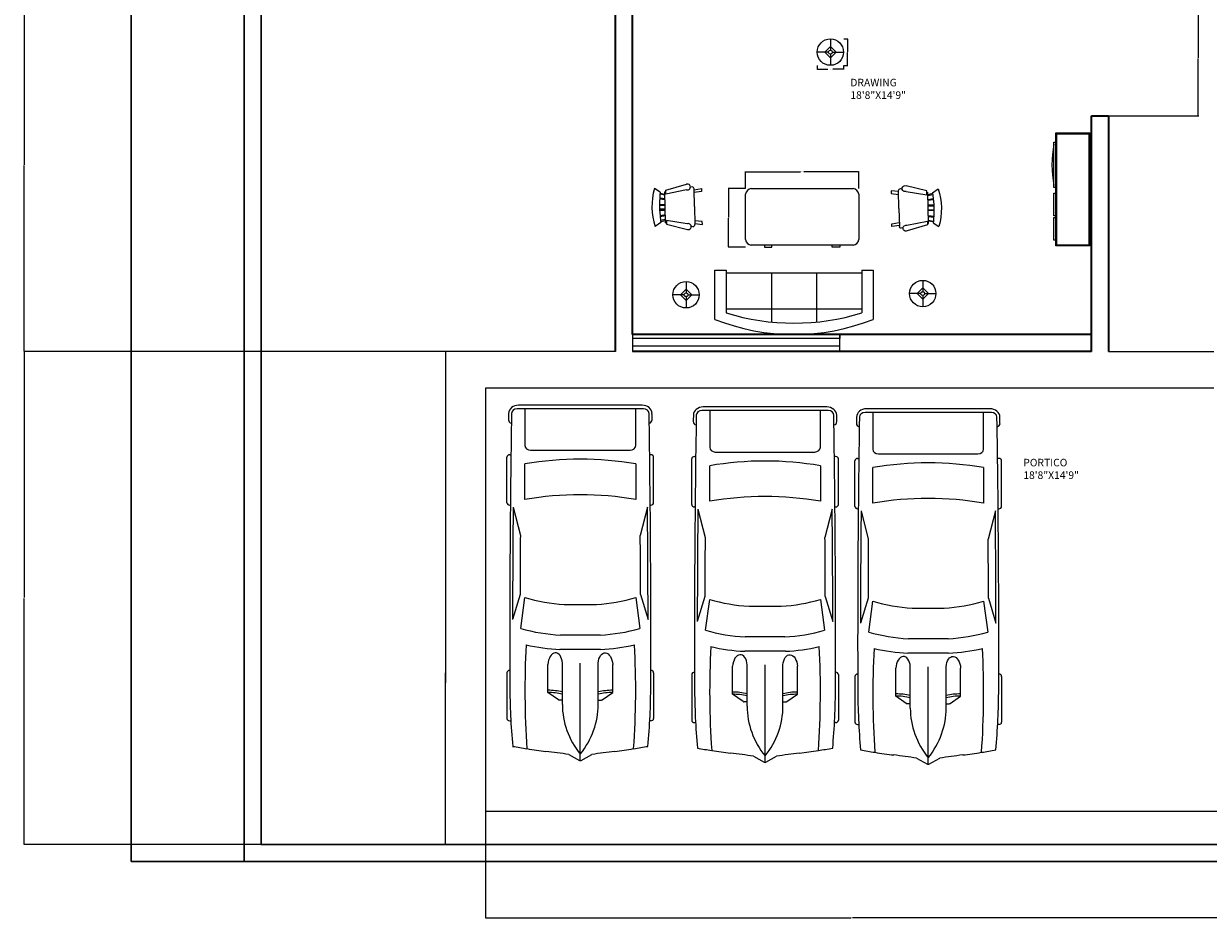
# Model space of a CAD drawing. Units: inches. Extents: x 727 to 1967, y -579 to 606.
# Tile 1 of 5: x 727 to 1355, y -552 to -78. Entities that reach past the tile are written whole.
import ezdxf

# ---------------------------------------------------------------- set-up
doc = ezdxf.new("R2010")
doc.units = ezdxf.units.IN
doc.header["$MEASUREMENT"] = 0
for name, color, linetype, lineweight in [('A-ANNO-DIMS', 2, 'Continuous', 18), ('A-AREA-IDEN', 7, 'Continuous', 18), ('A-FLOR-EXT', 7, 'Continuous', 25), ('A-FURN', 8, 'Continuous', 18), ('A-GLAZ', 4, 'Continuous', 18), ('A-WALL', 7, 'Continuous', 35), ('C-PKNG-VEHI', 8, 'Continuous', 13), ('C-PROP', 7, 'Continuous', 30)]:
    doc.layers.add(name, color=color, linetype=linetype, lineweight=lineweight)
doc.styles.get("Standard").update_dxf_attribs({"font": 'arial.ttf'})
doc.dimstyles.get("Standard").update_dxf_attribs({"dimtxt": 0.18, "dimasz": 0.18, "dimexe": 0.18, "dimexo": 0.0625, "dimgap": 0.09, "dimtad": 0, "dimtih": 1, "dimtoh": 1, "dimdec": 4, "dimzin": 0, "dimdsep": 46, "dimtxsty": 'Standard', "dimcen": 0.09, "dimadec": 0, "dimazin": 0, "dimtfac": 1, "dimtdec": 4, "dimtofl": 0, "dimtmove": 0, "dimatfit": 3, "dimfxl": 1, "dimtolj": 1, "dimtzin": 0, "dimarcsym": 0})

# ---------------------------------------------------------------- blocks, each defined once
blk = doc.blocks.new('Sofa - Roundback 7 ft.')
for p, q in [((-36.000027, -34), (-36.000027, -11.4696)), ((-12.00002, -32.4421), (-12.00003, -6.5971)), ((11.99997, -32.4421), (11.99998, -6.5971)), ((35.99998, -34), (35.99998, -11.4696)), ((-35.999844, -13.3819), (35.9998, -13.3819)), ((-36.000027, -32.4421), (35.99998, -32.4421))]:
    blk.add_line(p, q)
for points in [[(-36.000027, -34), (-42.000027, -34), (-42.000027, -8)], [(41.99998, -8), (41.99998, -34), (35.99998, -34)]]:
    blk.add_lwpolyline(points)
for centre, radius, start, end in [((0, -114.25), 114.25, 68.43141, 111.5686), ((-0.00001, -127.1968), 121.1968, 72.72033, 107.2797)]:
    blk.add_arc(centre, radius, start, end)
blk = doc.blocks.new('Chair - Rocking')
for p, q in [((-8, -4.5), (-10, -1.5)), ((-7.5, -4.5), (-7, -7)), ((-6.5, -7), (-7.02225, -4.43)), ((-4.5, -7), (-4.96674, -4.19951)), ((-4, -7), (-4.40532, -4.16272)), ((-1.5, -4.05012), (-1.5, -7)), ((-1, -7), (-1, -4.05012)), ((1, -7), (1, -4.04655)), ((1.5, -4.05012), (1.5, -7)), ((4, -7), (4.40187, -4.18694)), ((4.5, -7), (4.96761, -4.19437)), ((6.5, -7), (7, -4.4057)), ((7.5, -4.5), (7, -7)), ((8, -4.5), (10, -1.5)), ((-9, -7.5), (-12, -18.49999)), ((-7, -7.5), (-9, -7.5)), ((-9, -18.49999), (-7, -7.5)), ((-8.23428, -6.99939), (-8.3093, -7.47958)), ((-8.23041, -7), (8.23915, -7)), ((7, -7.5), (9, -7.5)), ((9, -18.49999), (7, -7.5)), ((8.31071, -7.48854), (8.23449, -7.00073)), ((9, -7.5), (12, -18.49999)), ((-10.36644, -20.64523), (-10.5, -21.49999)), ((-9, -22.49999), (-9.5, -26.49999)), ((0, -22.49999), (-9.5, -22.49999)), ((-8, -26.49999), (-7.5, -22.49999)), ((0, -22.49999), (9.5, -22.49999)), ((8, -26.49999), (7.5, -22.49999)), ((9, -22.49999), (9.5, -26.49999)), ((10.5, -21.49999), (10.3575, -20.58798)), ((-9.5, -26.49999), (-8, -26.49999)), ((9.5, -26.49999), (8, -26.49999))]:
    blk.add_line(p, q)
for centre, radius, start, end in [((0, -34.08333), 34.08333, 72.93847, 107.0615), ((0, -68.25004), 64.25, 93.92211, 97.15267), ((0, -68.25004), 64.25, 82.84733, 93.92211), ((-10.5, -18.99999), 1.58114, 161.5651, 18.43495), ((10.5, -18.99999), 1.58114, 161.5651, 18.43495), ((-9.5, -21.49999), 1, 180, 270), ((9.5, -21.49999), 1, 270, 0)]:
    blk.add_arc(centre, radius, start, end)
blk = doc.blocks.new('Lamp - Table')
for p, q in [((0, 7), (0, 1)), ((-1, 0), (-7, 0)), ((0, 3), (-3, 0)), ((-3, 0), (0, -3)), ((3, 0), (0, 3)), ((0, -3), (3, 0)), ((1, 0), (7, 0)), ((0, -1), (0, -7))]:
    blk.add_line(p, q)
for radius in [7, 1]:
    blk.add_circle((0, 0), radius)
blk = doc.blocks.new('Entertainment Center')
for p, q in [((-4, 0), (-5, -1)), ((4, 0), (-4, 0)), ((5, -1), (4, 0)), ((-17, -19), (-17, -1)), ((-17, -1), (43, -1)), ((-16.5, -18.5), (-16.5, -1.5)), ((-16.5, -1.5), (42.5, -1.5)), ((42.5, -1.5), (42.5, -18.5)), ((43, -1), (43, -19)), ((42.5, -18.5), (-16.5, -18.5)), ((43, -19), (-17, -19)), ((-12, -20), (-12, -19)), ((12, -20), (-12, -20)), ((12, -19), (12, -20)), ((15, -20), (15, -19)), ((27, -20), (15, -20)), ((27, -19), (27, -20)), ((28, -20), (28, -19)), ((40, -20), (28, -20)), ((40, -19), (40, -20))]:
    blk.add_line(p, q)
blk.add_arc((0, 40), 61, 259.6111, 280.3889)
blk = doc.blocks.new('Desk - 30 x 60 in.')
for p, q in [((-26.999995, 0), (26.999995, 0)), ((-29.999995, -27), (-29.999995, -3)), ((29.999995, -3), (29.999995, -27)), ((26.999995, -30), (-26.999995, -30)), ((-20.000005, -30), (-20.000005, -31)), ((-20.000005, -31), (-16.000005, -31)), ((-16.000005, -31), (-16.000005, -30)), ((15.999995, -31), (15.999995, -30)), ((19.999995, -31), (15.999995, -31)), ((19.999995, -30), (19.999995, -31))]:
    blk.add_line(p, q)
for centre, start, end in [((-26.499995, -3.5), 98.1301, 171.8699), ((26.499995, -3.5), 8.130102, 81.8699), ((-26.499995, -26.5), 188.1301, 261.8699), ((26.499995, -26.5), 278.1301, 351.8699)]:
    blk.add_arc(centre, 3.535534, start, end)
blk = doc.blocks.new('*U15')
for p, q in [((46.55, 38.89), (22.35, 38.89)), ((136.7, 38.89), (160.9, 38.89)), ((21.1, 37.41), (21.1, 36.83)), ((47.8, 37.39), (47.8, 37.41)), ((70.03, 31.54), (86.41, 29.35)), ((87.99, 31.87), (74.76, 35.92)), ((134.31, 35.6), (119.29, 31.78)), ((135.45, 37.07), (135.45, 37.41)), ((162.15, 37.41), (162.15, 36.77)), ((186.47, -33.5), (186.47, 33.5)), ((188.4, -32.76), (188.4, 32.76)), ((138.42, 29.35), (157.25, 29.35)), ((164.52, 26.39), (164.52, -26.39)), ((186.47, 29.35), (167.01, 29.35)), ((32.27, 11.63), (36.13, 17.17)), ((36.13, 17.17), (50.94, 17.17)), ((29.77, 9.51), (51.68, 9.51)), ((32.12, 9.51), (32.12, 11.15)), ((58.92, -10.77), (58.92, 10.77)), ((66.55, -10.53), (66.55, 10.53)), ((82.74, 8.5), (82.74, -8.5)), ((186.47, -10.53), (186.47, 10.53)), ((3.27, 6.13), (0.1, 0.41)), ((0, 0), (51.68, 0)), ((0.1, -0.41), (3.27, -6.13)), ((29.77, -9.51), (51.68, -9.51)), ((32.12, -9.51), (32.12, -11.15)), ((32.27, -11.63), (36.13, -17.17)), ((36.13, -17.17), (50.94, -17.17)), ((86.41, -29.35), (70.03, -31.54)), ((157.25, -29.35), (138.42, -29.35)), ((167.01, -29.35), (186.47, -29.35)), ((21.1, -37.41), (21.1, -36.83)), ((47.8, -37.39), (47.8, -37.41)), ((87.99, -31.87), (74.76, -35.92)), ((134.31, -35.6), (119.29, -31.78)), ((135.45, -37.07), (135.45, -37.41)), ((162.15, -37.41), (162.15, -36.77)), ((46.55, -38.89), (22.35, -38.89)), ((136.7, -38.89), (160.9, -38.89))]:
    blk.add_line(p, q)
for centre, major_axis, ratio, start_param, end_param in [((22.35, 37.41), (0, -1.48), 0.842304, 3.141593, 4.712389), ((46.55, 37.41), (0, 1.48), 0.842304, -1.570796, 0), ((136.7, 37.41), (0, -1.48), 0.842304, 3.141593, 4.712389), ((160.9, 37.41), (0, 1.48), 0.842304, -1.570796, 0), ((180.63, 35.84), (0, 2.22), 0.842304, -0.013017, 1.249894), ((64.48, -10556.36), (0, 10595.31), 0.842304, -0.013397, -0.013017), ((183.98, 32.76), (0, -5.25), 0.842304, 1.570796, 3.128196), ((266.03, -27.52), (0, 313.31), 0.842304, 1.367076, 1.39176), ((41.19, -490.86), (0, 528.23), 0.842304, 0.00281, 0.075598), ((64.48, -10555.62), (0, 10593.03), 0.842304, -0.013397, 0.002797), ((135.29, 5.39), (0, 81.77), 0.842304, 1.245306, 1.50788), ((64.48, -10555.62), (0, -10591.55), 0.842304, 3.133765, 3.140441), ((95.79, -3666.35), (0, -3698.24), 0.842304, 3.134049, 3.144098), ((183.98, 33.5), (0, -2.96), 0.842304, 1.570796, 3.128196), ((259.18, -27.52), (0, -305.3), 0.842304, 4.528606, 4.561838), ((37.47, -593.96), (0, -623.33), 0.842304, 3.096046, 3.200911), ((134.4, 5.39), (0, -89.78), 0.842304, 4.449482, 4.652344), ((149.6, 2.8), (0, -79.58), 0.842304, 4.372215, 4.640744), ((17.08, 0), (0, 147.02), 0.842304, 4.511394, 4.913384), ((35.91, 0), (0, 147.02), 0.842304, 4.511394, 4.913384), ((167.01, 26.39), (0, 2.96), 0.842304, 0, 1.570796), ((-204.49, 52.4), (0, -250.96), 0.842304, 1.385369, 1.434372), ((13.04, 17.01), (0, 27.42), 0.842304, 4.435146, 4.718221), ((14.2, 17.01), (0, 27.42), 0.842304, 4.435146, 4.718221), ((50.79, 13.34), (6.34, -0.36), 0.603834, -1.395552, 1.581315), ((29.77, -46.66), (0, 56.17), 0.842304, 0, 0.590319), ((32.75, 11.15), (0, 0.74), 0.842304, 0.879714, 1.570796), ((0.62, 0), (0, -0.74), 0.842304, 4.131459, 5.293319), ((-204.49, -52.4), (0, 250.96), 0.842304, -1.434372, -1.385369), ((29.77, 46.66), (0, 56.17), 0.842304, 2.551274, 3.141593), ((32.75, -11.15), (0, -0.74), 0.842304, 4.712389, 5.403472), ((13.04, -17.01), (0, -27.42), 0.842304, 1.564964, 1.848039), ((14.2, -17.01), (0, -27.42), 0.842304, 1.564964, 1.848039), ((134.4, -5.39), (0, -89.78), 0.842304, -1.510751, -1.307889), ((135.29, -5.39), (0, -81.77), 0.842304, -1.50788, -1.245306), ((149.6, -2.8), (0, -79.58), 0.842304, -1.499151, -1.230623), ((259.18, 27.52), (0, 305.3), 0.842304, 1.721348, 1.754579), ((266.03, 27.52), (0, 313.31), 0.842304, 1.749832, 1.774517), ((37.47, 593.96), (0, -623.33), 0.842304, -0.059319, 0.045547), ((167.01, -26.39), (0, -2.96), 0.842304, 4.712389, 6.283185), ((41.19, 490.86), (0, -528.23), 0.842304, -0.075598, -0.00281), ((22.35, -37.41), (0, 1.48), 0.842304, 1.570796, 3.141593), ((64.48, 10555.62), (0, 10593.03), 0.842304, 3.138796, 3.15499), ((46.55, -37.41), (0, -1.48), 0.842304, 0, 1.570796), ((64.48, 10555.62), (0, -10591.55), 0.842304, 0.001152, 0.007828), ((95.79, 3666.35), (0, -3698.24), 0.842304, -0.002505, 0.007544), ((136.7, -37.41), (0, -1.48), 0.842304, -1.570796, 0), ((160.9, -37.41), (0, 1.48), 0.842304, 3.141593, 4.712389), ((180.63, -35.84), (0, -2.22), 0.842304, -1.249894, 0.013017), ((183.98, -33.5), (0, 2.96), 0.842304, 3.15499, 4.712389), ((183.98, -32.76), (0, -5.25), 0.842304, 0.013397, 1.570796), ((64.48, 10556.36), (0, 10595.31), 0.842304, 3.15461, 3.15499)]:
    blk.add_ellipse(centre, major_axis=major_axis, ratio=ratio, start_param=start_param, end_param=end_param)
at = {"extrusion": (0, 0, -1)}
blk.add_ellipse((50.79, -13.34), major_axis=(6.34, 0.36), ratio=0.603834, start_param=-1.395552, end_param=1.581315, dxfattribs=at)
blk = doc.blocks.new('*D16')
at = {"layer": 'A-ANNO-DIMS', "color": 0, "lineweight": -2, "transparency": 16777216}
for p, q in [((1147.35, -99.9), (1147.35, -102.12)), ((1161.35, -99.9), (1161.35, -102.12)), ((1147.53, -101.94), (1153.01, -101.94)), ((1161.17, -101.94), (1155.69, -101.94))]:
    blk.add_line(p, q, dxfattribs=at)
at = {"layer": 'A-ANNO-DIMS', "color": 0, "transparency": 16777216}
for points in [[(1147.53, -101.91), (1147.53, -101.97), (1147.35, -101.94)], [(1161.17, -101.91), (1161.17, -101.97), (1161.35, -101.94)]]:
    blk.add_solid(points, dxfattribs=at)
at = {"layer": 'Defpoints', "color": 0, "transparency": 16777216}
for p in [(1147.35, -99.84), (1161.35, -99.84), (1161.35, -101.94)]:
    blk.add_point(p, dxfattribs=at)
at = {"layer": 'A-ANNO-DIMS', "color": 0, "transparency": 16777216, "insert": (1154.35, -101.94), "char_height": 0.18, "attachment_point": 5}
blk.add_mtext('\\A1;TABLE LAMP 14 TYP.', dxfattribs=at)
blk = doc.blocks.new('*D17')
at = {"layer": 'A-ANNO-DIMS', "color": 0, "lineweight": -2, "transparency": 16777216}
for p, q in [((1161.42, -85.84), (1163.63, -85.84)), ((1163.45, -86.02), (1163.45, -92.66)), ((1163.45, -99.66), (1163.45, -93.02)), ((1161.42, -99.84), (1163.63, -99.84))]:
    blk.add_line(p, q, dxfattribs=at)
at = {"layer": 'A-ANNO-DIMS', "color": 0, "transparency": 16777216}
for points in [[(1163.42, -86.02), (1163.48, -86.02), (1163.45, -85.84)], [(1163.42, -99.66), (1163.48, -99.66), (1163.45, -99.84)]]:
    blk.add_solid(points, dxfattribs=at)
at = {"layer": 'Defpoints', "color": 0, "transparency": 16777216}
for p in [(1161.35, -85.84), (1163.45, -85.84), (1161.35, -99.84)]:
    blk.add_point(p, dxfattribs=at)
at = {"layer": 'A-ANNO-DIMS', "color": 0, "transparency": 16777216, "insert": (1163.45, -92.84), "char_height": 0.18, "attachment_point": 5}
blk.add_mtext('\\A1;14 TYP.', dxfattribs=at)
blk = doc.blocks.new('*D26')
at = {"layer": 'A-ANNO-DIMS', "color": 0, "lineweight": -2, "transparency": 16777216}
for p, q in [((1109.4, -165.14), (1109.4, -156.02)), ((1109.58, -156.2), (1138.5, -156.2)), ((1169.22, -156.2), (1140.3, -156.2)), ((1169.4, -165.14), (1169.4, -156.02))]:
    blk.add_line(p, q, dxfattribs=at)
at = {"layer": 'A-ANNO-DIMS', "color": 0, "transparency": 16777216}
for points in [[(1109.58, -156.17), (1109.58, -156.23), (1109.4, -156.2)], [(1169.22, -156.17), (1169.22, -156.23), (1169.4, -156.2)]]:
    blk.add_solid(points, dxfattribs=at)
at = {"layer": 'Defpoints', "color": 0, "transparency": 16777216}
for p in [(1169.4, -156.2), (1109.4, -165.2), (1169.4, -165.2)]:
    blk.add_point(p, dxfattribs=at)
at = {"layer": 'A-ANNO-DIMS', "color": 0, "transparency": 16777216, "insert": (1139.4, -156.2), "char_height": 0.18, "attachment_point": 5}
blk.add_mtext('\\A1;DESK 60 TYP.', dxfattribs=at)
blk = doc.blocks.new('*D27')
at = {"layer": 'A-ANNO-DIMS', "color": 0, "lineweight": -2, "transparency": 16777216}
for p, q in [((1109.33, -165.2), (1100.22, -165.2)), ((1100.4, -165.38), (1100.4, -180.52)), ((1100.4, -196.02), (1100.4, -180.89)), ((1109.33, -196.2), (1100.22, -196.2))]:
    blk.add_line(p, q, dxfattribs=at)
at = {"layer": 'A-ANNO-DIMS', "color": 0, "transparency": 16777216}
for points in [[(1100.37, -165.38), (1100.43, -165.38), (1100.4, -165.2)], [(1100.37, -196.02), (1100.43, -196.02), (1100.4, -196.2)]]:
    blk.add_solid(points, dxfattribs=at)
at = {"layer": 'Defpoints', "color": 0, "transparency": 16777216}
for p in [(1100.4, -165.2), (1109.4, -165.2), (1109.4, -196.2)]:
    blk.add_point(p, dxfattribs=at)
at = {"layer": 'A-ANNO-DIMS', "color": 0, "transparency": 16777216, "insert": (1100.4, -180.7), "char_height": 0.18, "attachment_point": 5}
blk.add_mtext('\\A1;31 TYP.', dxfattribs=at)
blk = doc.blocks.new('*D48')
at = {"layer": 'A-ANNO-DIMS', "color": 0, "lineweight": -2, "transparency": 16777216}
for p, q in [((852.52, -53.98), (726.8, -53.98)), ((726.98, -54.16), (726.98, -152.55)), ((726.98, -251.3), (726.98, -152.92)), ((950.28, -251.48), (726.8, -251.48))]:
    blk.add_line(p, q, dxfattribs=at)
at = {"layer": 'A-ANNO-DIMS', "color": 0, "transparency": 16777216}
for points in [[(726.95, -54.16), (727.01, -54.16), (726.98, -53.98)], [(726.95, -251.3), (727.01, -251.3), (726.98, -251.48)]]:
    blk.add_solid(points, dxfattribs=at)
at = {"layer": 'Defpoints', "color": 0, "transparency": 16777216}
for p in [(852.58, -53.98), (726.98, -251.48), (950.34, -251.48)]:
    blk.add_point(p, dxfattribs=at)
at = {"layer": 'A-ANNO-DIMS', "color": 0, "transparency": 16777216, "insert": (726.98, -152.73), "char_height": 0.18, "attachment_point": 5}
blk.add_mtext('\\A1;197.5', dxfattribs=at)
blk = doc.blocks.new('*D49')
at = {"layer": 'A-ANNO-DIMS', "color": 0, "lineweight": -2, "transparency": 16777216}
for p, q in [((950.28, -251.48), (726.8, -251.48)), ((726.98, -251.66), (726.98, -381.97)), ((726.98, -512.63), (726.98, -382.33)), ((950.28, -512.81), (726.8, -512.81))]:
    blk.add_line(p, q, dxfattribs=at)
at = {"layer": 'A-ANNO-DIMS', "color": 0, "transparency": 16777216}
for points in [[(726.95, -251.66), (727.01, -251.66), (726.98, -251.48)], [(726.95, -512.63), (727.01, -512.63), (726.98, -512.81)]]:
    blk.add_solid(points, dxfattribs=at)
at = {"layer": 'Defpoints', "color": 0, "transparency": 16777216}
for p in [(950.34, -251.48), (726.98, -512.81), (950.34, -512.81)]:
    blk.add_point(p, dxfattribs=at)
at = {"layer": 'A-ANNO-DIMS', "color": 0, "transparency": 16777216, "insert": (726.98, -382.15), "char_height": 0.18, "attachment_point": 5}
blk.add_mtext('\\A1;261.3', dxfattribs=at)
blk = doc.blocks.new('*D50')
at = {"layer": 'A-ANNO-DIMS', "color": 0, "lineweight": -2, "transparency": 16777216}
for p, q in [((971.46, -495.19), (971.46, -551.9)), ((1360.08, -495.19), (1360.08, -551.9)), ((971.64, -551.72), (1165.38, -551.72)), ((1359.9, -551.72), (1166.17, -551.72))]:
    blk.add_line(p, q, dxfattribs=at)
at = {"layer": 'A-ANNO-DIMS', "color": 0, "transparency": 16777216}
for points in [[(971.64, -551.69), (971.64, -551.75), (971.46, -551.72)], [(1359.9, -551.69), (1359.9, -551.75), (1360.08, -551.72)]]:
    blk.add_solid(points, dxfattribs=at)
at = {"layer": 'Defpoints', "color": 0, "transparency": 16777216}
for p in [(971.46, -495.12), (1360.08, -495.12), (971.46, -551.72)]:
    blk.add_point(p, dxfattribs=at)
at = {"layer": 'A-ANNO-DIMS', "color": 0, "transparency": 16777216, "insert": (1165.77, -551.72), "char_height": 0.18, "attachment_point": 5}
blk.add_mtext('\\A1;388.6', dxfattribs=at)
blk = doc.blocks.new('*D59')
at = {"layer": 'A-ANNO-DIMS', "color": 0, "lineweight": -2, "transparency": 16777216}
for p, q in [((1292.91, -65.48), (1349.63, -65.48)), ((1349.45, -65.66), (1349.45, -95.86)), ((1349.45, -126.41), (1349.45, -96.22)), ((1292.91, -126.59), (1349.63, -126.59))]:
    blk.add_line(p, q, dxfattribs=at)
at = {"layer": 'A-ANNO-DIMS', "color": 0, "transparency": 16777216}
for points in [[(1349.42, -65.66), (1349.48, -65.66), (1349.45, -65.48)], [(1349.42, -126.41), (1349.48, -126.41), (1349.45, -126.59)]]:
    blk.add_solid(points, dxfattribs=at)
at = {"layer": 'Defpoints', "color": 0, "transparency": 16777216}
for p in [(1292.85, -65.48), (1292.85, -126.59), (1349.45, -126.59)]:
    blk.add_point(p, dxfattribs=at)
at = {"layer": 'A-ANNO-DIMS', "color": 0, "transparency": 16777216, "insert": (1349.45, -96.04), "char_height": 0.18, "attachment_point": 5}
blk.add_mtext('\\A1;61.1', dxfattribs=at)

msp = doc.modelspace()

# ---------------------------------------------------------------- linework, layer by layer
at = {"layer": 'A-FLOR-EXT'}
for p, q in [((1040.5236, -251.4849), (950.3408, -251.4849)), ((950.3408, -251.4849), (950.3408, -416.4849)), ((1301.8463, -251.4849), (1357.6449, -251.4849)), ((1357.6449, -270.8759), (971.4628, -270.8759)), ((971.4628, -270.8759), (971.4628, -491.2128)), ((950.3408, -416.4849), (950.3408, -427.1602)), ((950.3408, -512.8103), (950.3408, -421.8225)), ((971.4628, -491.2128), (971.4628, -495.1242)), ((971.4628, -495.1242), (1360.0813, -495.1242))]:
    msp.add_line(p, q, dxfattribs=at)
at = {"layer": 'A-GLAZ'}
for p, q in [((1049.5236, -242.4849), (1049.5236, -251.4849)), ((1159.3047, -244.6288), (1049.5236, -244.6288)), ((1049.5236, -244.6288), (1049.5236, -248.576)), ((1159.3047, -251.4849), (1159.3047, -242.4849)), ((1159.3047, -242.4849), (1159.3047, -244.6288)), ((1049.5236, -248.576), (1159.3047, -248.576)), ((1049.5236, -251.4849), (1159.3047, -251.4849))]:
    msp.add_line(p, q, dxfattribs=at)
at = {"layer": 'A-WALL'}
for p, q in [((1040.5236, -251.4849), (1040.5236, -53.9849)), ((1049.5236, -242.4849), (1049.5236, -65.4849)), ((1292.8463, -251.4849), (1292.8463, -126.5894)), ((1292.8463, -126.5894), (1301.8463, -126.5894)), ((1301.8463, -126.5894), (1301.8463, -251.4849)), ((1292.8463, -242.4849), (1049.5236, -242.4849)), ((1301.8463, -242.4186), (1301.8463, -251.4849)), ((1292.8463, -251.4849), (1049.5236, -251.4849))]:
    msp.add_line(p, q, dxfattribs=at)
at = {"layer": 'C-PROP'}
for p, q in [((783.5815, -461.8103), (783.5815, 392.0151)), ((843.5815, -521.8103), (843.5815, 299.0151)), ((852.5815, -512.8103), (852.5815, 299.0151)), ((783.5815, -521.8103), (783.5815, -461.8103)), ((1841.1781, -512.8103), (852.5815, -512.8103)), ((807.5815, -521.8103), (783.5815, -521.8103)), ((843.5815, -521.8103), (807.5815, -521.8103)), ((1850.1781, -521.8103), (843.5815, -521.8103))]:
    msp.add_line(p, q, dxfattribs=at)

# ---------------------------------------------------------------- block references
at = {"layer": 'A-FURN'}
for name, p in [('Lamp - Table', (1154.3526, -92.8357)), ('Desk - 30 x 60 in.', (1139.3974, -165.2048)), ('Lamp - Table', (1077.8408, -221.4273)), ('Lamp - Table', (1203.3262, -220.8096))]:
    msp.add_blockref(name, p, dxfattribs=at)
for name, p, rotation in [('Entertainment Center', (1292.8463, -152.5746), 270), ('Chair - Rocking', (1059.7917, -175.2314), 91.2499944704987), ('Sofa - Roundback 7 ft.', (1135.0726, -242.4849), 180)]:
    msp.add_blockref(name, p, dxfattribs=dict(at, rotation=rotation))
at = {"layer": 'A-FURN', "xscale": -1, "rotation": 271.2499944704995}
msp.add_blockref('Chair - Rocking', (1213.2257, -175.2314), dxfattribs=at)
at = {"layer": 'C-PKNG-VEHI', "rotation": 89.9999999999966}
for p in [(1021.7848, -468.3547), (1119.7271, -469.3042), (1206.2428, -470.2829)]:
    msp.add_blockref('*U15', p, dxfattribs=at)

# ---------------------------------------------------------------- texts
at = {"layer": 'A-AREA-IDEN', "char_height": 4, "attachment_point": 1}
for s, insert in [('DRAWING\\P18\'8"X14\'9"', (1164.9562, -106.9607)), ('PORTICO\\P18\'8"X14\'9"', (1256.6542, -308.3768))]:
    msp.add_mtext_dynamic_manual_height_columns(s, width=588.620786, gutter_width=1, heights=[0], dxfattribs=dict(at, insert=insert))

# ---------------------------------------------------------------- dimensions: what is measured, and where the dimension line sits
at = {"layer": 'A-ANNO-DIMS'}
for base, p1, p2, angle, picture, middle in [((726.9815, -251.4849), (852.5815, -53.9849), (950.3408, -251.4849), 90, '*D48', (726.9815, -152.7349)), ((1349.4463, -126.5894), (1292.8463, -65.4849), (1292.8463, -126.5894), 270, '*D59', (1349.4463, -96.0371)), ((726.9815, -512.8103), (950.3408, -251.4849), (950.3408, -512.8103), 90, '*D49', (726.9815, -382.1476)), ((971.4628, -551.7242), (1360.0813, -495.1242), (971.4628, -495.1242), 180, '*D50', (1165.7721, -551.7242))]:
    dim = msp.add_linear_dim(base=base, p1=p1, p2=p2, angle=angle, dimstyle='Standard', override={"dimdec": 1, "dimlfac": 1, "dimrnd": 0, "dimzin": 0, "dimdsep": 46, "dimlunit": 2}, dxfattribs=at)
    dim.commit()
    dim.dimension.update_dxf_attribs({"geometry": picture, "text_midpoint": middle})
for base, p1, p2, picture, middle in [((1163.4526, -85.8357), (1161.3526, -99.8357), (1161.3526, -85.8357), '*D17', (1163.4526, -92.8357)), ((1100.3974, -165.2048), (1109.3974, -196.2048), (1109.3974, -165.2048), '*D27', (1100.3974, -180.7048))]:
    dim = msp.add_linear_dim(base=base, p1=p1, p2=p2, angle=90, text='<> TYP.', dimstyle='Standard', override={"dimdec": 0, "dimlfac": 1, "dimrnd": 0, "dimzin": 0, "dimdsep": 46, "dimlunit": 2}, dxfattribs=at)
    dim.commit()
    dim.dimension.update_dxf_attribs({"geometry": picture, "text_midpoint": middle})
for base, p1, p2, text, picture, middle in [((1161.3526, -101.9357), (1147.3526, -99.8357), (1161.3526, -99.8357), 'TABLE LAMP <> TYP.', '*D16', (1154.3526, -101.9357)), ((1169.3974, -156.2048), (1109.3974, -165.2048), (1169.3974, -165.2048), 'DESK <> TYP.', '*D26', (1139.3974, -156.2048))]:
    dim = msp.add_linear_dim(base=base, p1=p1, p2=p2, text=text, dimstyle='Standard', override={"dimdec": 0, "dimlfac": 1, "dimrnd": 0, "dimzin": 0, "dimdsep": 46, "dimlunit": 2}, dxfattribs=at)
    dim.commit()
    dim.dimension.update_dxf_attribs({"geometry": picture, "text_midpoint": middle})

doc.saveas('drawing.dxf')
